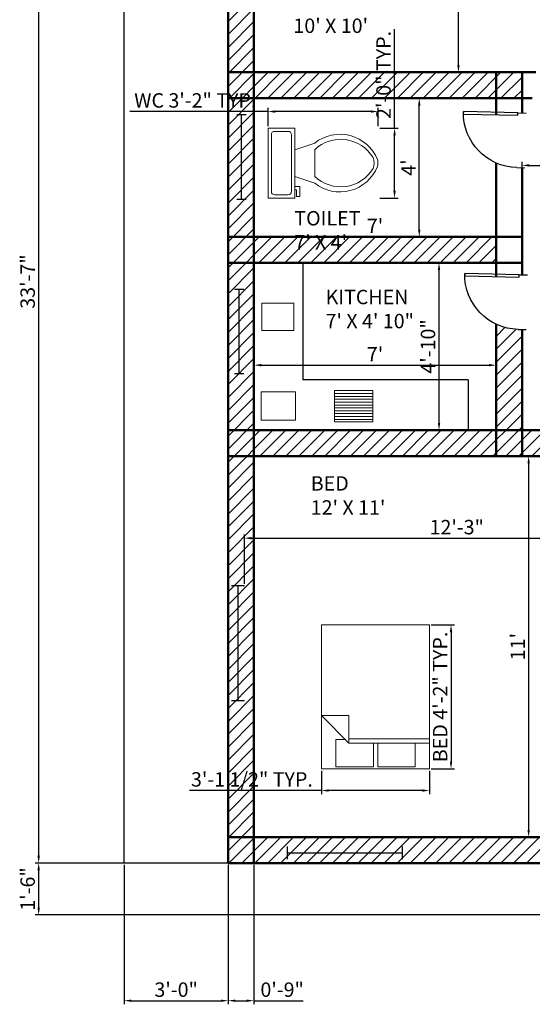
# Model space of a CAD drawing. Units: millimetres. Extents: x 2039 to 2694, y 890 to 1415.
# Tile 1 of 4: x 2039 to 2216, y 890 to 1232. Entities that reach past the tile are written whole.
import ezdxf

# ---------------------------------------------------------------- set-up
doc = ezdxf.new("R2010")
doc.units = ezdxf.units.MM
for name, color, linetype, lineweight in [('A-ANNO-DIMS', 80, 'Continuous', 18), ('A-AREA-IDEN', 130, 'Continuous', 25), ('A-FLOR-CASE', 140, 'Continuous', 25), ('A-FLOR-FIXT', 140, 'Continuous', 18), ('A-FLOR-FIXT-PATT', 140, 'Continuous', 13), ('A-WALL-PATT', 6, 'Continuous', 13), ('C-PROP', 200, 'Continuous', 25), ('doors', 10, 'Continuous', 25), ('furniture', 140, 'Continuous', 18), ('walls', 200, 'Continuous', 50), ('windows', 30, 'Continuous', 25)]:
    doc.layers.add(name, color=color, linetype=linetype, lineweight=lineweight)
doc.styles.get("Standard").update_dxf_attribs({"font": 'arial.ttf'})
doc.dimstyles.new('ISO-25', dxfattribs={"dimtxt": 5, "dimasz": 2.5, "dimexe": 1.25, "dimexo": 0.625, "dimtad": 1, "dimdec": 0, "dimlunit": 3, "dimtxsty": 'Standard', "dimcen": 2.5, "dimadec": 0, "dimazin": 0, "dimtfac": 1, "dimtdec": 0, "dimtmove": 0, "dimatfit": 3, "dimfxl": 1, "dimarcsym": 0})

# ---------------------------------------------------------------- blocks, each defined once
blk = doc.blocks.new('*U2')
for p, q in [((0, 0), (0, -6)), ((40, 0), (40, -6))]:
    blk.add_line(p, q)
blk.add_lwpolyline([(0, 0), (0, 40), (1.75, 40), (1.75, 0)], close=True)
blk.add_arc((0, 0), 40, 0, 90)
blk = doc.blocks.new('*U5')
for p, q in [((0, 4), (0, 0)), ((0, 2), (36, 2)), ((36, 4), (36, 0))]:
    blk.add_line(p, q)
blk = doc.blocks.new('*U4')
for p, q in [((0, 4), (0, 0)), ((36, 4), (36, 0)), ((0, 2), (36, 2))]:
    blk.add_line(p, q)
blk = doc.blocks.new('Bed - Queen')
for p, q in [((0, -80.00003), (0, 0)), ((0, 0), (59.99999, 0)), ((59.99999, 0), (59.99999, -80.00003)), ((7.99999, -1.2), (28.79998, -1.2)), ((7.99999, -14.4), (7.99999, -1.2)), ((28.79998, -1.2), (28.79998, -14.4)), ((31.19999, -1.2), (51.99999, -1.2)), ((31.19999, -14.4), (31.19999, -1.2)), ((51.99999, -1.2), (51.99999, -16.4)), ((0, -14.4), (44.8, -14.4)), ((59.99999, -29.6), (44.8, -14.4)), ((44.8, -14.4), (44.8, -29.6)), ((51.99999, -16.4), (46.79936, -16.4)), ((44.8, -16.8), (0, -16.8)), ((44.8, -29.6), (59.99999, -29.6)), ((59.99999, -80.00003), (0, -80.00003))]:
    blk.add_line(p, q)
blk = doc.blocks.new('Toilet - top')
for p, q in [((9.5, -6), (9.5, -2)), ((-10, -8.5), (-8, -8.5)), ((-10, -9.5), (-10, -8.5)), ((-8, -8.5), (-8, -8)), ((-7, -8), (-7, -9.5)), ((-4, -8), (-6, -14)), ((4, -8), (6, -14)), ((-7, -9.5), (-10, -9.5)), ((4, -14), (-4, -14))]:
    blk.add_line(p, q)
blk.add_lwpolyline([(10.5, -8), (10.5, 0), (-10.5, 0), (-10.5, -8)], close=True)
for points in [[(-9.5, -2), (-9.5, -6)], [(8.5, -1), (-8.5, -1)], [(-8.5, -7), (8.5, -7)]]:
    blk.add_lwpolyline(points)
for centre, radius, start, end in [((-8.62, -1.88), 0.884, 81.8699, 188.1301), ((8.62, -1.88), 0.884, 351.8699, 98.1301), ((-8.62, -6.12), 0.884, 171.8699, 278.1301), ((8.62, -6.12), 0.884, 261.8699, 8.1301), ((3.52, -21.58), 12.17, 141.4691, 247.9714), ((4.2, -21.82), 11.33, 136.3677, 238.9468), ((-3.52, -21.58), 12.17, 292.0284, 38.5307), ((-4.2, -21.82), 11.33, 301.053, 43.6321), ((0, -27.88), 4, 245.7318, 294.2682), ((0, -29), 4, 254.8605, 285.1395)]:
    blk.add_arc(centre, radius, start, end)
blk = doc.blocks.new('*D11')
at = {"layer": 'A-ANNO-DIMS', "color": 0, "lineweight": -2, "transparency": 16777216}
for p, q in [((2187.65, 1333.28), (2192.09, 1333.28)), ((2190.84, 1215.78), (2190.84, 1330.78)), ((2187.65, 1213.28), (2192.09, 1213.28))]:
    blk.add_line(p, q, dxfattribs=at)
at = {"layer": 'A-ANNO-DIMS', "color": 0, "transparency": 16777216}
for points in [[(2190.42, 1330.78), (2191.26, 1330.78), (2190.84, 1333.28)], [(2190.42, 1215.78), (2191.26, 1215.78), (2190.84, 1213.28)]]:
    blk.add_solid(points, dxfattribs=at)
at = {"layer": 'Defpoints', "color": 0, "transparency": 16777216}
for p in [(2187.03, 1333.28), (2190.84, 1333.28), (2187.03, 1213.28)]:
    blk.add_point(p, dxfattribs=at)
at = {"layer": 'A-ANNO-DIMS', "color": 0, "transparency": 16777216, "insert": (2187.66, 1273.28), "char_height": 5, "attachment_point": 5, "rotation": 90}
blk.add_mtext("10'", dxfattribs=at)
blk = doc.blocks.new('*D14')
at = {"layer": 'A-ANNO-DIMS', "color": 0, "lineweight": -2, "transparency": 16777216}
for p, q in [((2119.91, 1115.06), (2119.91, 1110.55)), ((2203.91, 1115.06), (2203.91, 1110.55)), ((2122.41, 1111.8), (2201.41, 1111.8))]:
    blk.add_line(p, q, dxfattribs=at)
at = {"layer": 'A-ANNO-DIMS', "color": 0, "transparency": 16777216}
for points in [[(2122.41, 1112.22), (2122.41, 1111.38), (2119.91, 1111.8)], [(2201.41, 1112.22), (2201.41, 1111.38), (2203.91, 1111.8)]]:
    blk.add_solid(points, dxfattribs=at)
at = {"layer": 'Defpoints', "color": 0, "transparency": 16777216}
for p in [(2119.91, 1115.68), (2203.91, 1115.68), (2203.91, 1111.8)]:
    blk.add_point(p, dxfattribs=at)
at = {"layer": 'A-ANNO-DIMS', "color": 0, "transparency": 16777216, "insert": (2161.91, 1114.93), "char_height": 5, "attachment_point": 5}
blk.add_mtext("7'", dxfattribs=at)
blk = doc.blocks.new('*D15')
at = {"layer": 'A-ANNO-DIMS', "color": 0, "lineweight": -2, "transparency": 16777216}
for p, q in [((2179.55, 1147.28), (2185.36, 1147.28)), ((2184.11, 1091.78), (2184.11, 1144.78)), ((2179.55, 1089.28), (2185.36, 1089.28))]:
    blk.add_line(p, q, dxfattribs=at)
at = {"layer": 'A-ANNO-DIMS', "color": 0, "transparency": 16777216}
for points in [[(2183.69, 1144.78), (2184.53, 1144.78), (2184.11, 1147.28)], [(2183.69, 1091.78), (2184.53, 1091.78), (2184.11, 1089.28)]]:
    blk.add_solid(points, dxfattribs=at)
at = {"layer": 'Defpoints', "color": 0, "transparency": 16777216}
for p in [(2178.93, 1147.28), (2184.11, 1147.28), (2178.93, 1089.28)]:
    blk.add_point(p, dxfattribs=at)
at = {"layer": 'A-ANNO-DIMS', "color": 0, "transparency": 16777216, "insert": (2180.93, 1118.28), "char_height": 5, "attachment_point": 5, "rotation": 90}
blk.add_mtext('4\'-10"', dxfattribs=at)
blk = doc.blocks.new('*D16')
at = {"layer": 'A-ANNO-DIMS', "color": 0, "lineweight": -2, "transparency": 16777216}
for p, q in [((2119.91, 1161.58), (2119.91, 1155.03)), ((2203.91, 1161.56), (2203.91, 1155.03)), ((2122.41, 1156.28), (2201.41, 1156.28))]:
    blk.add_line(p, q, dxfattribs=at)
at = {"layer": 'A-ANNO-DIMS', "color": 0, "transparency": 16777216}
for points in [[(2122.41, 1156.69), (2122.41, 1155.86), (2119.91, 1156.28)], [(2201.41, 1156.69), (2201.41, 1155.86), (2203.91, 1156.28)]]:
    blk.add_solid(points, dxfattribs=at)
at = {"layer": 'Defpoints', "color": 0, "transparency": 16777216}
for p in [(2119.91, 1162.2), (2203.91, 1162.19), (2203.91, 1156.28)]:
    blk.add_point(p, dxfattribs=at)
at = {"layer": 'A-ANNO-DIMS', "color": 0, "transparency": 16777216, "insert": (2161.91, 1159.4), "char_height": 5, "attachment_point": 5}
blk.add_mtext("7'", dxfattribs=at)
blk = doc.blocks.new('*D17')
at = {"layer": 'A-ANNO-DIMS', "color": 0, "lineweight": -2, "transparency": 16777216}
for p, q in [((2180.58, 1204.28), (2176.01, 1204.28)), ((2177.26, 1158.78), (2177.26, 1201.78)), ((2180.58, 1156.28), (2176.01, 1156.28))]:
    blk.add_line(p, q, dxfattribs=at)
at = {"layer": 'A-ANNO-DIMS', "color": 0, "transparency": 16777216}
for points in [[(2176.84, 1201.78), (2177.67, 1201.78), (2177.26, 1204.28)], [(2176.84, 1158.78), (2177.67, 1158.78), (2177.26, 1156.28)]]:
    blk.add_solid(points, dxfattribs=at)
at = {"layer": 'Defpoints', "color": 0, "transparency": 16777216}
for p in [(2177.26, 1204.28), (2181.21, 1204.28), (2181.21, 1156.28)]:
    blk.add_point(p, dxfattribs=at)
at = {"layer": 'A-ANNO-DIMS', "color": 0, "transparency": 16777216, "insert": (2174.13, 1180.28), "char_height": 5, "attachment_point": 5, "rotation": 90}
blk.add_mtext("4'", dxfattribs=at)
blk = doc.blocks.new('*D18')
at = {"layer": 'A-ANNO-DIMS', "color": 0, "lineweight": -2, "transparency": 16777216}
for p, q in [((2212.91, 1162.32), (2212.91, 1182.29)), ((2215.41, 1181.04), (2366.41, 1181.04)), ((2368.91, 1162.32), (2368.91, 1182.29))]:
    blk.add_line(p, q, dxfattribs=at)
at = {"layer": 'A-ANNO-DIMS', "color": 0, "transparency": 16777216}
for points in [[(2215.41, 1181.46), (2215.41, 1180.62), (2212.91, 1181.04)], [(2366.41, 1181.46), (2366.41, 1180.62), (2368.91, 1181.04)]]:
    blk.add_solid(points, dxfattribs=at)
at = {"layer": 'Defpoints', "color": 0, "transparency": 16777216}
for p in [(2368.91, 1181.04), (2212.91, 1161.69), (2368.91, 1161.69)]:
    blk.add_point(p, dxfattribs=at)
at = {"layer": 'A-ANNO-DIMS', "color": 0, "transparency": 16777216, "insert": (2290.91, 1184.22), "char_height": 5, "attachment_point": 5}
blk.add_mtext("13'", dxfattribs=at)
blk = doc.blocks.new('*D22')
at = {"layer": 'A-ANNO-DIMS', "color": 0, "lineweight": -2, "transparency": 16777216}
for p, q in [((2116.59, 1036.07), (2116.59, 1053.1)), ((2119.09, 1051.85), (2261.41, 1051.85)), ((2263.91, 1036.07), (2263.91, 1053.1))]:
    blk.add_line(p, q, dxfattribs=at)
at = {"layer": 'A-ANNO-DIMS', "color": 0, "transparency": 16777216}
for points in [[(2119.09, 1052.27), (2119.09, 1051.44), (2116.59, 1051.85)], [(2261.41, 1052.27), (2261.41, 1051.44), (2263.91, 1051.85)]]:
    blk.add_solid(points, dxfattribs=at)
at = {"layer": 'Defpoints', "color": 0, "transparency": 16777216}
for p in [(2263.91, 1051.85), (2116.59, 1035.45), (2263.91, 1035.45)]:
    blk.add_point(p, dxfattribs=at)
at = {"layer": 'A-ANNO-DIMS', "color": 0, "transparency": 16777216, "insert": (2190.25, 1055.03), "char_height": 5, "attachment_point": 5}
blk.add_mtext('12\'-3"', dxfattribs=at)
blk = doc.blocks.new('*D23')
at = {"layer": 'A-ANNO-DIMS', "color": 0, "lineweight": -2, "transparency": 16777216}
for p, q in [((2204.53, 1080.28), (2216.45, 1080.28)), ((2215.2, 1077.78), (2215.2, 950.78)), ((2204.53, 948.28), (2216.45, 948.28))]:
    blk.add_line(p, q, dxfattribs=at)
at = {"layer": 'A-ANNO-DIMS', "color": 0, "transparency": 16777216}
for points in [[(2214.78, 1077.78), (2215.62, 1077.78), (2215.2, 1080.28)], [(2214.78, 950.78), (2215.62, 950.78), (2215.2, 948.28)]]:
    blk.add_solid(points, dxfattribs=at)
at = {"layer": 'Defpoints', "color": 0, "transparency": 16777216}
for p in [(2203.91, 1080.28), (2203.91, 948.28), (2215.2, 948.28)]:
    blk.add_point(p, dxfattribs=at)
at = {"layer": 'A-ANNO-DIMS', "color": 0, "transparency": 16777216, "insert": (2212.07, 1014.28), "char_height": 5, "attachment_point": 5, "rotation": 90}
blk.add_mtext("11'", dxfattribs=at)
blk = doc.blocks.new('*D29')
at = {"layer": 'A-ANNO-DIMS', "color": 0, "lineweight": -2, "transparency": 16777216}
for p, q in [((2181.42, 1021.78), (2189.52, 1021.78)), ((2188.27, 1019.28), (2188.27, 974.39)), ((2181.42, 971.89), (2189.52, 971.89))]:
    blk.add_line(p, q, dxfattribs=at)
at = {"layer": 'A-ANNO-DIMS', "color": 0, "transparency": 16777216}
for points in [[(2187.86, 1019.28), (2188.69, 1019.28), (2188.27, 1021.78)], [(2187.86, 974.39), (2188.69, 974.39), (2188.27, 971.89)]]:
    blk.add_solid(points, dxfattribs=at)
at = {"layer": 'Defpoints', "color": 0, "transparency": 16777216}
for p in [(2180.79, 1021.78), (2180.79, 971.89), (2188.27, 971.89)]:
    blk.add_point(p, dxfattribs=at)
at = {"layer": 'A-ANNO-DIMS', "color": 0, "transparency": 16777216, "insert": (2185.14, 996.83), "char_height": 5, "attachment_point": 5, "rotation": 90}
blk.add_mtext('BED 4\'-2" TYP.', dxfattribs=at)
blk = doc.blocks.new('*D30')
at = {"layer": 'A-ANNO-DIMS', "color": 0, "lineweight": -2, "transparency": 16777216}
for p, q in [((2143.37, 971.26), (2143.37, 963.16)), ((2180.79, 971.26), (2180.79, 963.16)), ((2143.37, 964.41), (2097.5, 964.41)), ((2178.29, 964.41), (2145.87, 964.41))]:
    blk.add_line(p, q, dxfattribs=at)
at = {"layer": 'A-ANNO-DIMS', "color": 0, "transparency": 16777216}
for points in [[(2145.87, 964.82), (2145.87, 963.99), (2143.37, 964.41)], [(2178.29, 964.82), (2178.29, 963.99), (2180.79, 964.41)]]:
    blk.add_solid(points, dxfattribs=at)
at = {"layer": 'Defpoints', "color": 0, "transparency": 16777216}
for p in [(2143.37, 971.89), (2180.79, 971.89), (2143.37, 964.41)]:
    blk.add_point(p, dxfattribs=at)
at = {"layer": 'A-ANNO-DIMS', "color": 0, "transparency": 16777216, "insert": (2119.19, 967.62), "char_height": 5, "attachment_point": 5}
blk.add_mtext('3\'-1 1/2" TYP.', dxfattribs=at)
blk = doc.blocks.new('*D31')
at = {"layer": 'A-ANNO-DIMS', "color": 0, "lineweight": -2, "transparency": 16777216}
for p, q in [((2124.81, 1199.69), (2076.8, 1199.69)), ((2124.81, 1194.59), (2124.81, 1200.94)), ((2160.46, 1199.69), (2127.31, 1199.69)), ((2162.96, 1194.59), (2162.96, 1200.94))]:
    blk.add_line(p, q, dxfattribs=at)
at = {"layer": 'A-ANNO-DIMS', "color": 0, "transparency": 16777216}
for points in [[(2127.31, 1200.11), (2127.31, 1199.27), (2124.81, 1199.69)], [(2160.46, 1200.11), (2160.46, 1199.27), (2162.96, 1199.69)]]:
    blk.add_solid(points, dxfattribs=at)
at = {"layer": 'Defpoints', "color": 0, "transparency": 16777216}
for p in [(2124.81, 1199.69), (2124.81, 1193.97), (2162.96, 1193.97)]:
    blk.add_point(p, dxfattribs=at)
at = {"layer": 'A-ANNO-DIMS', "color": 0, "transparency": 16777216, "insert": (2099.55, 1202.9), "char_height": 5, "attachment_point": 5}
blk.add_mtext('WC 3\'-2" TYP.', dxfattribs=at)
blk = doc.blocks.new('*D32')
at = {"layer": 'A-ANNO-DIMS', "color": 0, "lineweight": -2, "transparency": 16777216}
for p, q in [((2168.69, 1193.97), (2168.69, 1228.28)), ((2163.59, 1193.97), (2169.94, 1193.97)), ((2168.69, 1172.22), (2168.69, 1191.47)), ((2163.59, 1169.72), (2169.94, 1169.72))]:
    blk.add_line(p, q, dxfattribs=at)
at = {"layer": 'A-ANNO-DIMS', "color": 0, "transparency": 16777216}
for points in [[(2168.27, 1191.47), (2169.1, 1191.47), (2168.69, 1193.97)], [(2168.27, 1172.22), (2169.1, 1172.22), (2168.69, 1169.72)]]:
    blk.add_solid(points, dxfattribs=at)
at = {"layer": 'Defpoints', "color": 0, "transparency": 16777216}
for p in [(2162.96, 1193.97), (2168.69, 1193.97), (2162.96, 1169.72)]:
    blk.add_point(p, dxfattribs=at)
at = {"layer": 'A-ANNO-DIMS', "color": 0, "transparency": 16777216, "insert": (2165.51, 1212.37), "char_height": 5, "attachment_point": 5, "rotation": 90}
blk.add_mtext('2\'-0" TYP.', dxfattribs=at)
blk = doc.blocks.new('*D36')
at = {"layer": 'A-ANNO-DIMS', "color": 0, "lineweight": -2, "transparency": 16777216}
for p, q in [((2110.28, 1342.28), (2043.96, 1342.28)), ((2045.21, 941.78), (2045.21, 1339.78)), ((2110.28, 939.28), (2043.96, 939.28))]:
    blk.add_line(p, q, dxfattribs=at)
at = {"layer": 'A-ANNO-DIMS', "color": 0, "transparency": 16777216}
for points in [[(2044.79, 1339.78), (2045.62, 1339.78), (2045.21, 1342.28)], [(2044.79, 941.78), (2045.62, 941.78), (2045.21, 939.28)]]:
    blk.add_solid(points, dxfattribs=at)
at = {"layer": 'Defpoints', "color": 0, "transparency": 16777216}
for p in [(2045.21, 1342.28), (2110.91, 1342.28), (2110.91, 939.28)]:
    blk.add_point(p, dxfattribs=at)
at = {"layer": 'A-ANNO-DIMS', "color": 0, "transparency": 16777216, "insert": (2042.03, 1140.78), "char_height": 5, "attachment_point": 5, "rotation": 90}
blk.add_mtext('33\'-7"', dxfattribs=at)
blk = doc.blocks.new('*D39')
at = {"layer": 'A-ANNO-DIMS', "color": 0, "lineweight": -2, "transparency": 16777216}
for p, q in [((2408.28, 939.28), (2043.96, 939.28)), ((2045.21, 923.78), (2045.21, 936.78)), ((2408.28, 921.28), (2043.96, 921.28))]:
    blk.add_line(p, q, dxfattribs=at)
at = {"layer": 'A-ANNO-DIMS', "color": 0, "transparency": 16777216}
for points in [[(2044.79, 936.78), (2045.62, 936.78), (2045.21, 939.28)], [(2044.79, 923.78), (2045.62, 923.78), (2045.21, 921.28)]]:
    blk.add_solid(points, dxfattribs=at)
at = {"layer": 'Defpoints', "color": 0, "transparency": 16777216}
for p in [(2045.21, 939.28), (2408.91, 939.28), (2408.91, 921.28)]:
    blk.add_point(p, dxfattribs=at)
at = {"layer": 'A-ANNO-DIMS', "color": 0, "transparency": 16777216, "insert": (2042.03, 930.28), "char_height": 5, "attachment_point": 5, "rotation": 90}
blk.add_mtext('1\'-6"', dxfattribs=at)
blk = doc.blocks.new('*D41')
at = {"layer": 'A-ANNO-DIMS', "color": 0, "lineweight": -2, "transparency": 16777216}
for p, q in [((2074.91, 938.65), (2074.91, 890.33)), ((2110.91, 938.65), (2110.91, 890.33)), ((2077.41, 891.58), (2108.41, 891.58))]:
    blk.add_line(p, q, dxfattribs=at)
at = {"layer": 'A-ANNO-DIMS', "color": 0, "transparency": 16777216}
for points in [[(2077.41, 891.99), (2077.41, 891.16), (2074.91, 891.58)], [(2108.41, 891.99), (2108.41, 891.16), (2110.91, 891.58)]]:
    blk.add_solid(points, dxfattribs=at)
at = {"layer": 'Defpoints', "color": 0, "transparency": 16777216}
for p in [(2074.91, 939.28), (2110.91, 939.28), (2110.91, 891.58)]:
    blk.add_point(p, dxfattribs=at)
at = {"layer": 'A-ANNO-DIMS', "color": 0, "transparency": 16777216, "insert": (2092.91, 894.76), "char_height": 5, "attachment_point": 5}
blk.add_mtext('3\'-0"', dxfattribs=at)
blk = doc.blocks.new('*D42')
at = {"layer": 'A-ANNO-DIMS', "color": 0, "lineweight": -2, "transparency": 16777216}
for p, q in [((2110.91, 938.65), (2110.91, 890.33)), ((2119.91, 938.65), (2119.91, 890.33)), ((2113.41, 891.58), (2117.41, 891.58)), ((2119.91, 891.58), (2136.95, 891.58))]:
    blk.add_line(p, q, dxfattribs=at)
at = {"layer": 'A-ANNO-DIMS', "color": 0, "transparency": 16777216}
for points in [[(2113.41, 891.99), (2113.41, 891.16), (2110.91, 891.58)], [(2117.41, 891.99), (2117.41, 891.16), (2119.91, 891.58)]]:
    blk.add_solid(points, dxfattribs=at)
at = {"layer": 'Defpoints', "color": 0, "transparency": 16777216}
for p in [(2110.91, 939.28), (2119.91, 939.28), (2119.91, 891.58)]:
    blk.add_point(p, dxfattribs=at)
at = {"layer": 'A-ANNO-DIMS', "color": 0, "transparency": 16777216, "insert": (2129.68, 894.75), "char_height": 5, "attachment_point": 5}
blk.add_mtext('0\'-9"', dxfattribs=at)

msp = doc.modelspace()

# ---------------------------------------------------------------- hatches: boundary and pattern name
at = {"layer": 'A-FLOR-FIXT-PATT'}
h = msp.add_hatch(dxfattribs=at)
h.set_pattern_fill('ANSI31', color=256, scale=0.3149606, angle=-45, style=0)
h.paths.add_polyline_path([(2147.88, 1103.04), (2161.14, 1103.04), (2161.14, 1092.12), (2147.88, 1092.12)])
at = {"layer": 'A-WALL-PATT'}
h = msp.add_hatch(dxfattribs=at)
h.set_pattern_fill('ANSI31', color=256)
h.paths.add_polyline_path([(2119.91, 1333.28), (2110.91, 1333.28), (2110.91, 1213.28), (2119.91, 1213.28)])
h.paths.add_polyline_path([(2119.91, 1342.28), (2110.91, 1342.28), (2110.91, 1333.28), (2119.91, 1333.28)])
h.paths.add_polyline_path([(2239.91, 1342.28), (2119.91, 1342.28), (2119.91, 1333.28), (2239.91, 1333.28)])
h.paths.add_polyline_path([(2368.91, 1342.28), (2248.91, 1342.28), (2248.91, 1333.28), (2368.91, 1333.28)])
h.paths.add_polyline_path([(2248.91, 1342.28), (2239.91, 1342.28), (2239.91, 1333.28), (2248.91, 1333.28)])
h.paths.add_polyline_path([(2248.91, 1333.28), (2239.91, 1333.28), (2239.91, 1213.28), (2248.91, 1213.28)])
h.paths.add_polyline_path([(2203.91, 1213.28), (2119.91, 1213.28), (2119.91, 1204.28), (2203.91, 1204.28)])
h.paths.add_polyline_path([(2119.91, 1204.28), (2110.91, 1204.28), (2110.91, 1156.28), (2119.91, 1156.28)])
h.paths.add_polyline_path([(2119.91, 1213.28), (2110.91, 1213.28), (2110.91, 1204.28), (2119.91, 1204.28)])
h.paths.add_polyline_path([(2212.91, 1213.28), (2203.91, 1213.28), (2203.91, 1204.28), (2212.91, 1204.28)])
h.paths.add_polyline_path([(2368.91, 1213.28), (2273.37, 1213.28, -0.081603), (2274.54, 1206.12), (2274.54, 1204.28), (2368.91, 1204.28)])
h.paths.add_polyline_path([(2377.91, 1333.28), (2368.91, 1333.28), (2368.91, 1213.28), (2377.91, 1213.28)])
h.paths.add_polyline_path([(2617.91, 1342.28), (2377.91, 1342.28), (2377.91, 1333.28), (2617.91, 1333.28)])
h.paths.add_polyline_path([(2377.91, 1342.28), (2368.91, 1342.28), (2368.91, 1333.28), (2377.91, 1333.28)])
h.paths.add_polyline_path([(2626.91, 1333.28), (2617.91, 1333.28), (2617.91, 948.28), (2626.91, 948.28)])
h.paths.add_polyline_path([(2377.91, 1204.28), (2368.91, 1204.28), (2368.91, 1156.28), (2377.91, 1156.28)])
h.paths.add_polyline_path([(2377.91, 1156.28), (2368.91, 1156.28), (2368.91, 1147.28), (2377.91, 1147.28)])
h.paths.add_polyline_path([(2377.91, 1213.28), (2368.91, 1213.28), (2368.91, 1204.28), (2377.91, 1204.28)])
h.paths.add_polyline_path([(2368.91, 1156.28), (2360.56, 1156.28), (2360.56, 1148.39), (2360.56, 1147.28), (2368.91, 1147.28)])
h.paths.add_polyline_path([(2399.91, 1156.28), (2377.91, 1156.28), (2377.91, 1147.28), (2399.91, 1147.28)])
h.paths.add_polyline_path([(2408.91, 1156.28), (2399.91, 1156.28), (2399.91, 1147.28), (2408.91, 1147.28)])
h.paths.add_polyline_path([(2339.63, 1156.28), (2327.91, 1156.28), (2327.91, 1147.28), (2338.19, 1147.28), (2338.19, 1148.39, -0.090365)])
h.paths.add_polyline_path([(2327.91, 1156.28), (2318.91, 1156.28), (2318.91, 1147.28), (2327.91, 1147.28)])
h.paths.add_polyline_path([(2327.91, 1147.28), (2318.91, 1147.28), (2318.91, 1041.28), (2327.91, 1041.28)])
h.paths.add_polyline_path([(2408.91, 1109.51), (2399.91, 1109.51), (2399.91, 948.28), (2408.91, 948.28)])
h.paths.add_polyline_path([(2272.91, 1080.28), (2263.91, 1080.28), (2263.91, 1041.28), (2272.91, 1041.28)])
h.paths.add_polyline_path([(2272.91, 1089.28), (2263.91, 1089.28), (2263.91, 1080.28), (2272.91, 1080.28)])
h.paths.add_polyline_path([(2263.91, 1089.28), (2252.09, 1089.28), (2252.48, 1080.28), (2263.91, 1080.28)])
h.paths.add_polyline_path([(2229.75, 1088.3), (2229.7, 1089.28), (2212.91, 1089.28), (2212.91, 1080.28), (2231.62, 1080.28, -0.092884)])
h.paths.add_polyline_path([(2212.91, 1124.18), (2211.56, 1124.21, -0.10492), (2203.91, 1126.01), (2203.91, 1089.28), (2212.91, 1089.28)])
h.paths.add_polyline_path([(2212.91, 1089.28), (2203.91, 1089.28), (2203.91, 1080.28), (2212.91, 1080.28)])
h.paths.add_polyline_path([(2203.91, 1089.28), (2119.91, 1089.28), (2119.91, 1080.28), (2203.91, 1080.28)])
h.paths.add_polyline_path([(2119.91, 1147.28), (2110.91, 1147.28), (2110.91, 1089.28), (2119.91, 1089.28)])
h.paths.add_polyline_path([(2119.91, 1156.28), (2110.91, 1156.28), (2110.91, 1147.28), (2119.91, 1147.28)])
h.paths.add_polyline_path([(2203.91, 1156.28), (2119.91, 1156.28), (2119.91, 1147.28), (2136.91, 1147.28), (2203.91, 1147.28)])
h.paths.add_polyline_path([(2119.91, 1080.28), (2110.91, 1080.28), (2110.91, 948.28), (2119.91, 948.28)])
h.paths.add_polyline_path([(2119.91, 1089.28), (2110.91, 1089.28), (2110.91, 1080.28), (2119.91, 1080.28)])
h.paths.add_polyline_path([(2119.91, 948.28), (2110.91, 948.28), (2110.91, 939.28), (2119.91, 939.28)])
h.paths.add_polyline_path([(2263.91, 948.28), (2119.91, 948.28), (2119.91, 939.28), (2263.91, 939.28)])
h.paths.add_polyline_path([(2318.91, 948.28), (2272.91, 948.28), (2272.91, 939.28), (2318.91, 939.28)])
h.paths.add_polyline_path([(2272.91, 948.28), (2263.91, 948.28), (2263.91, 939.28), (2272.91, 939.28)])
h.paths.add_polyline_path([(2272.91, 1041.28), (2263.91, 1041.28), (2263.91, 1032.28), (2272.91, 1032.28)])
h.paths.add_polyline_path([(2327.91, 1032.28), (2318.91, 1032.28), (2318.91, 948.28), (2327.91, 948.28)])
h.paths.add_polyline_path([(2399.91, 948.28), (2327.91, 948.28), (2327.91, 939.28), (2399.91, 939.28)])
h.paths.add_polyline_path([(2327.91, 948.28), (2318.91, 948.28), (2318.91, 939.28), (2327.91, 939.28)])
h.paths.add_polyline_path([(2408.91, 948.28), (2399.91, 948.28), (2399.91, 939.28), (2408.91, 939.28)])
h.paths.add_polyline_path([(2617.91, 948.28), (2408.91, 948.28), (2408.91, 939.28), (2617.91, 939.28)])
h.paths.add_polyline_path([(2626.91, 948.28), (2617.91, 948.28), (2617.91, 939.28), (2626.91, 939.28)])
h.paths.add_polyline_path([(2132.32, 1149.06), (2159.44, 1149.06), (2159.44, 1167.69), (2132.32, 1167.69)], flags=9)

# ---------------------------------------------------------------- linework, layer by layer
at = {"layer": 'A-FLOR-CASE'}
for p, q in [((2119.91, 1147.28), (2136.91, 1147.28)), ((2136.91, 1147.28), (2136.91, 1106.68)), ((2194.24, 1106.68), (2136.91, 1106.68)), ((2194.24, 1106.68), (2194.24, 1089.28)), ((2203.91, 1089.28), (2203.91, 1106.68))]:
    msp.add_line(p, q, dxfattribs=at)
at = {"layer": 'A-FLOR-FIXT'}
for points in [[(2122.58, 1133.32), (2133.73, 1133.32), (2133.73, 1123.86), (2122.58, 1123.86)], [(2122.45, 1102.59), (2134.3, 1102.59), (2134.3, 1092.74), (2122.45, 1092.74)], [(2147.88, 1103.04), (2161.14, 1103.04), (2161.14, 1092.12), (2147.88, 1092.12)]]:
    msp.add_lwpolyline(points, close=True, dxfattribs=at)
at = {"layer": 'C-PROP'}
for p, q in [((2074.91, 939.28), (2074.91, 1304.98)), ((2110.91, 939.28), (2074.91, 939.28))]:
    msp.add_line(p, q, dxfattribs=at)
at = {"layer": 'walls'}
for p, q in [((2110.91, 1342.28), (2110.91, 939.28)), ((2119.91, 1342.28), (2119.91, 939.28)), ((2110.91, 1213.28), (2217.66, 1213.28)), ((2203.91, 1213.28), (2203.91, 1198.57)), ((2212.91, 1213.28), (2212.91, 1199.21)), ((2110.91, 1204.28), (2216.48, 1204.28)), ((2203.91, 1181.88), (2203.91, 1142.49)), ((2212.91, 1180.26), (2212.91, 1143.12)), ((2110.91, 1156.28), (2212.91, 1156.28)), ((2110.91, 1147.28), (2212.91, 1147.28)), ((2203.91, 1126.01), (2203.91, 1080.28)), ((2212.91, 1124.18), (2212.91, 1080.28)), ((2110.91, 1089.28), (2229.7, 1089.28)), ((2110.91, 1080.28), (2231.62, 1080.28)), ((2110.91, 948.28), (2626.91, 948.28)), ((2110.91, 939.28), (2626.91, 939.28))]:
    msp.add_line(p, q, dxfattribs=at)

# ---------------------------------------------------------------- block references
at = {"layer": 'A-FLOR-FIXT', "xscale": 1.154546597564434, "yscale": 1.154546597564434, "zscale": 1.154546597564434, "rotation": 90}
msp.add_blockref('Toilet - top', (2124.81, 1181.84), dxfattribs=at)
at = {"layer": 'doors', "xscale": -0.4735158435176222, "yscale": 0.4735158435176223, "zscale": 0.4735158435176223, "rotation": 88.74685468085674}
for p in [(2211.49, 1199.24), (2211.97, 1143.14)]:
    msp.add_blockref('*U2', p, dxfattribs=at)
at = {"layer": 'furniture', "xscale": 0.6236252200436019, "yscale": 0.6236252200436019, "zscale": 0.6236252200436019, "rotation": 180}
msp.add_blockref('Bed - Queen', (2180.79, 971.89), dxfattribs=at)
at = {"layer": 'windows', "rotation": 90}
for name, p, xscale, yscale, zscale in [('*U5', (2117.25, 1169.31), 0.8142679173318405, 0.8142679173318405, 0.8142679173318405), ('*U5', (2116.43, 1108.87), 0.8142679173318405, 0.8142679173318405, 0.8142679173318405), ('*U4', (2116.59, 995.56), 1.108036427899419, 1.108036427899419, 1.108036427899419)]:
    msp.add_blockref(name, p, dxfattribs=dict(at, xscale=xscale, yscale=yscale, zscale=zscale))
at = {"layer": 'windows', "xscale": 1.108036427899419, "yscale": 1.108036427899419, "zscale": 1.108036427899419}
msp.add_blockref('*U4', (2131.41, 940.57), dxfattribs=at)

# ---------------------------------------------------------------- texts
at = {"layer": 'A-AREA-IDEN', "char_height": 5, "attachment_point": 1}
for s, width, insert in [("BEDROOM\\P10' X 10'", 49.8516, (2133.59, 1240.25)), ("TOILET\\P7' X 4' ", 38.8495, (2133.9, 1165.21)), ('KITCHEN\\P7\' X 4\' 10"', 30.8019, (2144.75, 1137.92)), ("BED \\P12' X 11'", 58.1079, (2139.6, 1073.33))]:
    msp.add_mtext_dynamic_manual_height_columns(s, width=width, gutter_width=12.5, heights=[0], dxfattribs=dict(at, insert=insert))

# ---------------------------------------------------------------- dimensions: what is measured, and where the dimension line sits
at = {"layer": 'A-ANNO-DIMS'}
for base, p1, p2, override, picture, middle in [((2045.21, 1342.28), (2110.91, 939.28), (2110.91, 1342.28), {"dimdec": 1, "dimlfac": 1, "dimrnd": 0, "dimzin": 1, "dimdsep": 46, "dimlunit": 4, "dimfrac": 2}, '*D36', (2042.03, 1140.78)), ((2190.84, 1333.28), (2187.03, 1213.28), (2187.03, 1333.28), {"dimclrd": 0, "dimclre": 0, "dimclrt": 0}, '*D11', (2187.66, 1273.28)), ((2177.26, 1204.28), (2181.21, 1156.28), (2181.21, 1204.28), {"dimclrd": 0, "dimclre": 0, "dimclrt": 0}, '*D17', (2174.13, 1180.28)), ((2184.11, 1147.28), (2178.93, 1089.28), (2178.93, 1147.28), {"dimclrd": 0, "dimclre": 0, "dimclrt": 0}, '*D15', (2180.93, 1118.28)), ((2215.2, 948.28), (2203.91, 1080.28), (2203.91, 948.28), {"dimclrd": 0, "dimclre": 0, "dimclrt": 0}, '*D23', (2212.07, 1014.28)), ((2045.21, 939.28), (2408.91, 921.28), (2408.91, 939.28), {"dimdec": 1, "dimlfac": 1, "dimrnd": 0, "dimzin": 1, "dimdsep": 46, "dimlunit": 4, "dimfrac": 2}, '*D39', (2042.03, 930.28))]:
    dim = msp.add_linear_dim(base=base, p1=p1, p2=p2, angle=90, dimstyle='ISO-25', override=override, dxfattribs=at)
    dim.commit()
    dim.dimension.update_dxf_attribs({"geometry": picture, "text_midpoint": middle})
for base, p1, p2, angle, text, picture, middle in [((2168.6852, 1193.9661), (2162.9622, 1169.7206), (2162.9622, 1193.9661), 90, '<> TYP.', '*D32', (2165.5074, 1212.3724)), ((2124.8088, 1199.6891), (2162.9622, 1193.9661), (2124.8088, 1193.9661), 180, 'WC <> TYP.', '*D31', (2099.5538, 1202.901)), ((2188.27, 971.89), (2180.79, 1021.78), (2180.79, 971.89), 270, 'BED <> TYP.', '*D29', (2185.14, 996.83)), ((2143.37, 964.41), (2180.79, 971.89), (2143.37, 971.89), 180, '<> TYP.', '*D30', (2119.19, 967.62))]:
    dim = msp.add_linear_dim(base=base, p1=p1, p2=p2, angle=angle, text=text, dimstyle='ISO-25', override={"dimdec": 1, "dimlfac": 1, "dimrnd": 0, "dimzin": 1, "dimdsep": 46, "dimlunit": 4, "dimfrac": 2}, dxfattribs=at)
    dim.commit()
    dim.dimension.update_dxf_attribs({"geometry": picture, "text_midpoint": middle})
for base, p1, p2, override, picture, middle in [((2368.91, 1181.04), (2212.91, 1161.69), (2368.91, 1161.69), {"dimclrd": 0, "dimclre": 0, "dimclrt": 0}, '*D18', (2290.91, 1184.22)), ((2203.91, 1156.28), (2119.91, 1162.2), (2203.91, 1162.19), {"dimclrd": 0, "dimclre": 0, "dimclrt": 0}, '*D16', (2161.91, 1159.4)), ((2203.91, 1111.8), (2119.91, 1115.68), (2203.91, 1115.68), {"dimclrd": 0, "dimclre": 0, "dimclrt": 0}, '*D14', (2161.91, 1114.93)), ((2263.91, 1051.85), (2116.59, 1035.45), (2263.91, 1035.45), {"dimclrd": 0, "dimclre": 0, "dimclrt": 0}, '*D22', (2190.25, 1055.03)), ((2110.91, 891.58), (2074.91, 939.28), (2110.91, 939.28), {"dimdec": 1, "dimlfac": 1, "dimrnd": 0, "dimzin": 1, "dimdsep": 46, "dimlunit": 4, "dimfrac": 2}, '*D41', (2092.91, 894.76)), ((2119.91, 891.58), (2110.91, 939.28), (2119.91, 939.28), {"dimdec": 1, "dimlfac": 1, "dimrnd": 0, "dimzin": 1, "dimdsep": 46, "dimlunit": 4, "dimfrac": 2}, '*D42', (2129.68, 894.75))]:
    dim = msp.add_linear_dim(base=base, p1=p1, p2=p2, dimstyle='ISO-25', override=override, dxfattribs=at)
    dim.commit()
    dim.dimension.update_dxf_attribs({"geometry": picture, "text_midpoint": middle})

doc.saveas('drawing.dxf')
